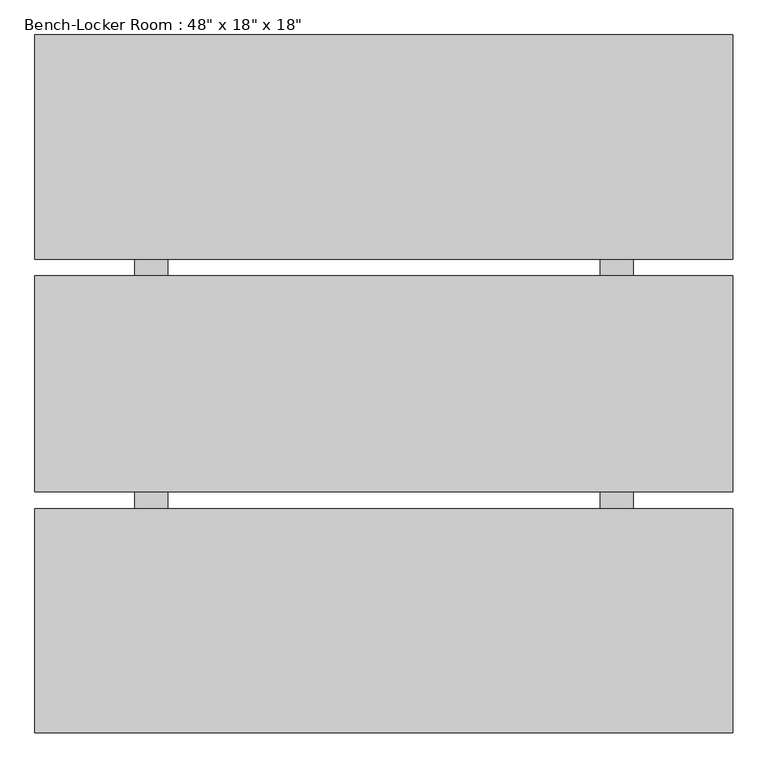
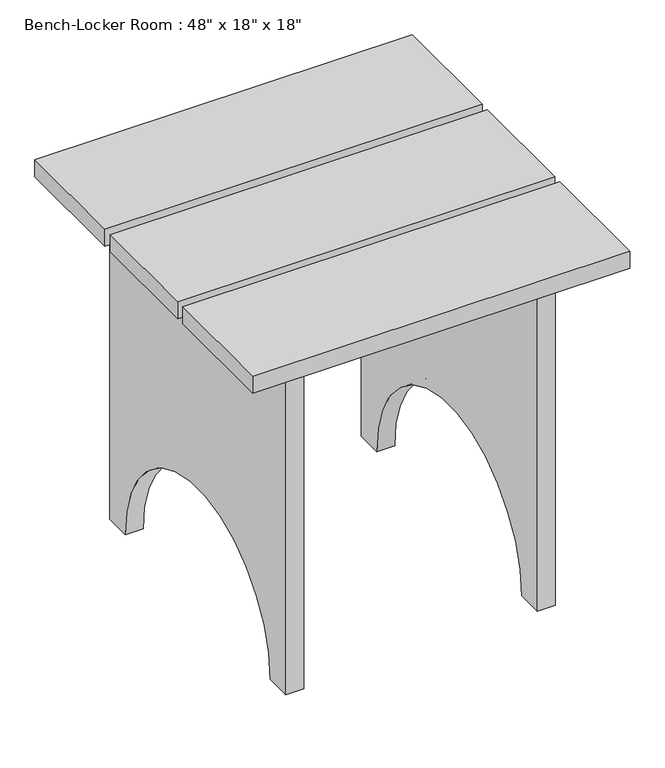
"""IFC4 building model written with IfcOpenShell, lengths in millimetres: furniture geometry."""

from ifc_helpers import new_model, si_unit, point, frame, frame_2d, origin, place, context, project, spatial, polyline, circle_curve, trimmed, segment, composite_curve, outline, extrude, source, transform, mapped, element, save


def furniture_92cb3fd8(model_context):
    return source(origin(), model_context, "Body", "SweptSolid", [
        extrude(outline(polyline([(378.0852459, 352.6852459), (378.0852459, 9.7852459), (-688.7147541, 9.7852459), (-688.7147541, 352.6852459), (378.0852459, 352.6852459)])), frame((0.0, 0.0, 1016.0), z_axis=(0.0, 0.0, 1.0), x_axis=(1.0, 0.0, 0.0)), (0.0, 0.0, 1.0), 50.8),
        extrude(outline(polyline([(378.0852459, -714.1147541), (-688.7147541, -714.1147541), (-688.7147541, -371.2147541), (378.0852459, -371.2147541), (378.0852459, -714.1147541)])), frame((0.0, 0.0, 1016.0), z_axis=(0.0, 0.0, 1.0), x_axis=(1.0, 0.0, 0.0)), (0.0, 0.0, 1.0), 50.8),
        extrude(outline(polyline([(378.0852459, -15.6147541), (378.0852459, -345.8147541), (-688.7147541, -345.8147541), (-688.7147541, -15.6147541), (378.0852459, -15.6147541)])), frame((0.0, 0.0, 1016.0), z_axis=(0.0, 0.0, 1.0), x_axis=(1.0, 0.0, 0.0)), (0.0, 0.0, 1.0), 50.8),
        extrude(outline(composite_curve([segment(polyline([(251.0852459, 0.0), (174.8852459, 0.0)]), True, "CONTINUOUS"), segment(trimmed(circle_curve(frame_2d((-180.7147541, 0.0)), 355.6), [point((174.8852459, 0.0))], [point((-536.3147541, 0.0))], True, "CARTESIAN"), True, "CONTINUOUS"), segment(polyline([(-536.3147541, 0.0), (-612.5147541, 0.0), (-612.5147541, 1016.0), (251.0852459, 1016.0), (251.0852459, 0.0)]), True, "CONTINUOUS")], self_intersect=False)), frame((-536.3147541, 0.0, 0.0), z_axis=(1.0, 0.0, 0.0), x_axis=(0.0, 1.0, 0.0)), (0.0, 0.0, 1.0), 50.8),
        extrude(outline(composite_curve([segment(polyline([(-612.5147541, 0.0), (-612.5147541, 1016.0), (251.0852459, 1016.0), (251.0852459, 0.0), (174.8852459, 0.0)]), True, "CONTINUOUS"), segment(trimmed(circle_curve(frame_2d((-180.7147541, 0.0)), 355.6), [point((174.8852459, 0.0))], [point((-536.3147541, 0.0))], True, "CARTESIAN"), True, "CONTINUOUS"), segment(polyline([(-536.3147541, 0.0), (-612.5147541, 0.0)]), True, "CONTINUOUS")], self_intersect=False)), frame((174.8852459, 0.0, 0.0), z_axis=(1.0, 0.0, 0.0), x_axis=(0.0, 1.0, 0.0)), (0.0, 0.0, 1.0), 50.8),
    ])


if __name__ == "__main__":
    model = new_model("IFC4")
    model_context = context("Model", 3, world=origin())
    ifc_project = project(units=[si_unit("LENGTHUNIT", "METRE", prefix="MILLI")], contexts=[model_context])
    site = spatial("IfcSite", under=ifc_project)
    building = spatial("IfcBuilding", under=site)
    placement = place(None, origin())
    furniture_shape = furniture_92cb3fd8(model_context)
    element("IfcFurniture", 1, ObjectType="Bench-Locker Room : 48\" x 18\" x 18\"", at=placement, inside=building, context=model_context, shape_type="MappedRepresentation", body=[
        mapped(furniture_shape, transform((0.0, 0.0, 0.0), x_axis=(1.0, 0.0, 0.0), y_axis=(0.0, 1.0, 0.0), z_axis=(0.0, 0.0, 1.0))),
    ])
    save(model, "model.ifc")

# Revit data of these elements
# Type "Bench-Locker Room : 48\" x 18\" x 18\""
#   Assembly Code = "E2020200"
#   Depth = 3' - 6"
#   Height = 3' - 6"
#   Width = 3' - 6"
#   Bench Material = Cherry
#   Default Elevation = 0
# Element 1 (IfcFurniture, "Bench-Locker Room : 48\" x 18\" x 18\"")
#   Materials on its faces: "Cherry"
# Materials
#   "Cherry": class "Wood", colour RGB 226 177 128, transparency 0, Description = "Prunus Serotina", Cost = 0
